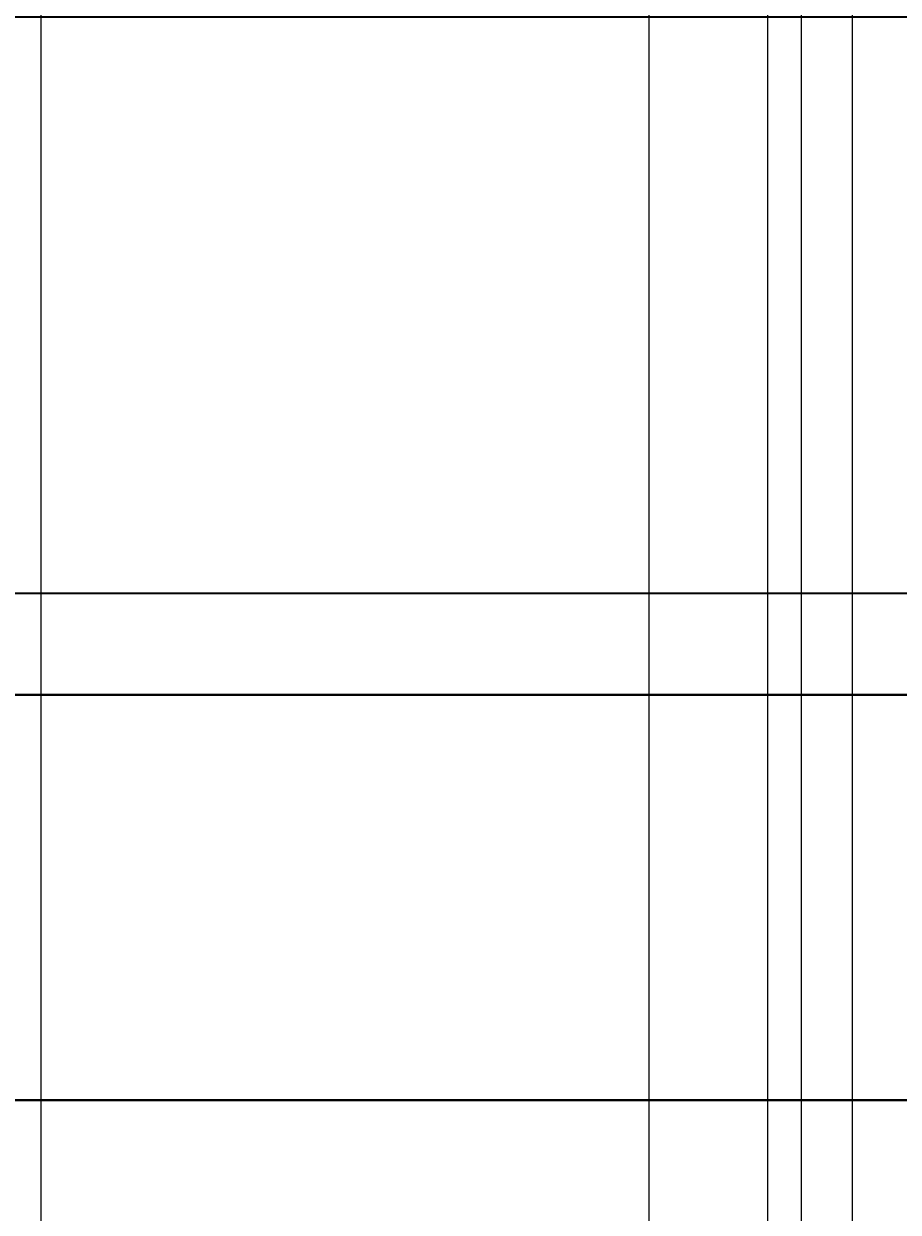
# Model space of a CAD drawing. Units: inches. Extents: x -6 to 289, y -8 to 323.
# Tile 63 of 107: x 212 to 238, y 124 to 159. Entities that reach past the tile are written whole.
import ezdxf

# ---------------------------------------------------------------- set-up
doc = ezdxf.new("R2010")
doc.units = ezdxf.units.IN
doc.header["$MEASUREMENT"] = 0
doc.layers.add('A-ANNO-DIMS', color=2, linetype='Continuous', lineweight=18)
doc.layers.add('A-ELEV', color=7, linetype='Continuous', lineweight=35)
doc.styles.get("Standard").update_dxf_attribs({"font": 'arial.ttf'})
doc.dimstyles.get("Standard").update_dxf_attribs({"dimtxt": 0.18, "dimasz": 0.18, "dimexe": 0.18, "dimexo": 0.0625, "dimgap": 0.09, "dimtad": 0, "dimtih": 1, "dimtoh": 1, "dimdec": 4, "dimzin": 0, "dimdsep": 46, "dimtxsty": 'Standard', "dimcen": 0.09, "dimadec": 0, "dimazin": 0, "dimtfac": 1, "dimtdec": 4, "dimtofl": 0, "dimtmove": 0, "dimatfit": 3, "dimfxl": 1, "dimtolj": 1, "dimtzin": 0, "dimarcsym": 0})

# ---------------------------------------------------------------- blocks, each defined once
blk = doc.blocks.new('*D24')
at = {"layer": 'A-ANNO-DIMS', "color": 0, "lineweight": -2, "transparency": 16777216}
for p, q in [((126.946, 178.654), (288.653, 178.654)), ((288.473, 178.474), (288.473, 159.153)), ((288.473, 139.469), (288.473, 158.789)), ((259.226, 139.289), (288.653, 139.289))]:
    blk.add_line(p, q, dxfattribs=at)
at = {"layer": 'A-ANNO-DIMS', "color": 0, "transparency": 16777216}
for points in [[(288.443, 178.474), (288.503, 178.474), (288.473, 178.654)], [(288.443, 139.469), (288.503, 139.469), (288.473, 139.289)]]:
    blk.add_solid(points, dxfattribs=at)
at = {"layer": 'Defpoints', "color": 0, "transparency": 16777216}
for p in [(126.883, 178.654), (288.473, 178.654), (259.164, 139.289)]:
    blk.add_point(p, dxfattribs=at)
at = {"layer": 'A-ANNO-DIMS', "color": 0, "transparency": 16777216, "insert": (288.473, 158.971), "char_height": 0.18, "attachment_point": 5}
blk.add_mtext('\\A1;39.365', dxfattribs=at)
blk = doc.blocks.new('*D43')
at = {"layer": 'A-ANNO-DIMS', "color": 0, "lineweight": -2, "transparency": 16777216}
for p, q in [((211.292, 224.326), (211.292, -8.391)), ((212.292, 224.326), (212.292, -8.391)), ((211.472, -8.211), (211.669, -8.211)), ((212.112, -8.211), (211.915, -8.211))]:
    blk.add_line(p, q, dxfattribs=at)
at = {"layer": 'A-ANNO-DIMS', "color": 0, "transparency": 16777216}
for points in [[(211.472, -8.181), (211.472, -8.241), (211.292, -8.211)], [(212.112, -8.181), (212.112, -8.241), (212.292, -8.211)]]:
    blk.add_solid(points, dxfattribs=at)
at = {"layer": 'Defpoints', "color": 0, "transparency": 16777216}
for p in [(211.292, 224.389), (212.292, 224.389), (212.292, -8.211)]:
    blk.add_point(p, dxfattribs=at)
at = {"layer": 'A-ANNO-DIMS', "color": 0, "transparency": 16777216, "insert": (211.792, -8.211), "char_height": 0.18, "attachment_point": 5}
blk.add_mtext('\\A1;1', dxfattribs=at)
blk = doc.blocks.new('*D44')
at = {"layer": 'A-ANNO-DIMS', "color": 0, "lineweight": -2, "transparency": 16777216}
for p, q in [((212.292, 224.326), (212.292, -8.391)), ((233.792, 224.326), (233.792, -8.391)), ((212.472, -8.211), (222.716, -8.211)), ((233.612, -8.211), (223.368, -8.211))]:
    blk.add_line(p, q, dxfattribs=at)
at = {"layer": 'A-ANNO-DIMS', "color": 0, "transparency": 16777216}
for points in [[(212.472, -8.181), (212.472, -8.241), (212.292, -8.211)], [(233.612, -8.181), (233.612, -8.241), (233.792, -8.211)]]:
    blk.add_solid(points, dxfattribs=at)
at = {"layer": 'Defpoints', "color": 0, "transparency": 16777216}
for p in [(212.292, 224.389), (233.792, 224.389), (233.792, -8.211)]:
    blk.add_point(p, dxfattribs=at)
at = {"layer": 'A-ANNO-DIMS', "color": 0, "transparency": 16777216, "insert": (223.042, -8.211), "char_height": 0.18, "attachment_point": 5}
blk.add_mtext('\\A1;21.5', dxfattribs=at)
blk = doc.blocks.new('*D45')
at = {"layer": 'A-ANNO-DIMS', "color": 0, "lineweight": -2, "transparency": 16777216}
for p, q in [((234.792, 225.326), (234.792, -8.391)), ((233.792, 224.326), (233.792, -8.391)), ((233.972, -8.211), (234.169, -8.211)), ((234.612, -8.211), (234.415, -8.211))]:
    blk.add_line(p, q, dxfattribs=at)
at = {"layer": 'A-ANNO-DIMS', "color": 0, "transparency": 16777216}
for points in [[(233.972, -8.181), (233.972, -8.241), (233.792, -8.211)], [(234.612, -8.181), (234.612, -8.241), (234.792, -8.211)]]:
    blk.add_solid(points, dxfattribs=at)
at = {"layer": 'Defpoints', "color": 0, "transparency": 16777216}
for p in [(234.792, 225.389), (233.792, 224.389), (234.792, -8.211)]:
    blk.add_point(p, dxfattribs=at)
at = {"layer": 'A-ANNO-DIMS', "color": 0, "transparency": 16777216, "insert": (234.292, -8.211), "char_height": 0.18, "attachment_point": 5}
blk.add_mtext('\\A1;1', dxfattribs=at)
blk = doc.blocks.new('*D46')
at = {"layer": 'A-ANNO-DIMS', "color": 0, "lineweight": -2, "transparency": 16777216}
for p, q in [((236.292, 226.826), (236.292, -8.391)), ((234.792, 225.326), (234.792, -8.391)), ((234.972, -8.211), (235.296, -8.211)), ((236.112, -8.211), (235.788, -8.211))]:
    blk.add_line(p, q, dxfattribs=at)
at = {"layer": 'A-ANNO-DIMS', "color": 0, "transparency": 16777216}
for points in [[(234.972, -8.181), (234.972, -8.241), (234.792, -8.211)], [(236.112, -8.181), (236.112, -8.241), (236.292, -8.211)]]:
    blk.add_solid(points, dxfattribs=at)
at = {"layer": 'Defpoints', "color": 0, "transparency": 16777216}
for p in [(236.292, 226.889), (234.792, 225.389), (236.292, -8.211)]:
    blk.add_point(p, dxfattribs=at)
at = {"layer": 'A-ANNO-DIMS', "color": 0, "transparency": 16777216, "insert": (235.542, -8.211), "char_height": 0.18, "attachment_point": 5}
blk.add_mtext('\\A1;1.5', dxfattribs=at)
blk = doc.blocks.new('*D80')
at = {"layer": 'A-ANNO-DIMS', "color": 0, "lineweight": -2, "transparency": 16777216}
for p, q in [((188.292, 116.842), (188.292, 322.969)), ((230.292, 116.842), (230.292, 322.969)), ((188.472, 322.789), (209.07, 322.789)), ((230.112, 322.789), (209.513, 322.789))]:
    blk.add_line(p, q, dxfattribs=at)
at = {"layer": 'A-ANNO-DIMS', "color": 0, "transparency": 16777216}
for points in [[(188.472, 322.819), (188.472, 322.759), (188.292, 322.789)], [(230.112, 322.819), (230.112, 322.759), (230.292, 322.789)]]:
    blk.add_solid(points, dxfattribs=at)
at = {"layer": 'Defpoints', "color": 0, "transparency": 16777216}
for p in [(230.292, 322.789), (188.292, 116.779), (230.292, 116.779)]:
    blk.add_point(p, dxfattribs=at)
at = {"layer": 'A-ANNO-DIMS', "color": 0, "transparency": 16777216, "insert": (209.292, 322.789), "char_height": 0.18, "attachment_point": 5}
blk.add_mtext('\\A1;42', dxfattribs=at)
blk = doc.blocks.new('*D81')
at = {"layer": 'A-ANNO-DIMS', "color": 0, "lineweight": -2, "transparency": 16777216}
for p, q in [((230.292, 68.842), (230.292, 322.969)), ((245.215, 66.286), (245.215, 322.969)), ((230.472, 322.789), (237.298, 322.789)), ((245.035, 322.789), (238.208, 322.789))]:
    blk.add_line(p, q, dxfattribs=at)
at = {"layer": 'A-ANNO-DIMS', "color": 0, "transparency": 16777216}
for points in [[(230.472, 322.819), (230.472, 322.759), (230.292, 322.789)], [(245.035, 322.819), (245.035, 322.759), (245.215, 322.789)]]:
    blk.add_solid(points, dxfattribs=at)
at = {"layer": 'Defpoints', "color": 0, "transparency": 16777216}
for p in [(245.215, 322.789), (230.292, 68.779), (245.215, 66.224)]:
    blk.add_point(p, dxfattribs=at)
at = {"layer": 'A-ANNO-DIMS', "color": 0, "transparency": 16777216, "insert": (237.753, 322.789), "char_height": 0.18, "attachment_point": 5}
blk.add_mtext('\\A1;14.923', dxfattribs=at)

msp = doc.modelspace()

# ---------------------------------------------------------------- linework, layer by layer
at = {"layer": 'A-ELEV'}
for p, q in [((115.1638, 139.2888), (259.1638, 139.2888)), ((259.1638, 127.2888), (115.1638, 127.2888)), ((115.1638, 127.2888), (259.1638, 127.2888))]:
    msp.add_line(p, q, dxfattribs=at)
for points in [[(247.1638, 139.2888), (115.1638, 139.2888), (115.1638, 162.3484), (247.1638, 162.3484)], [(244.1638, 142.2888), (118.1638, 142.2888), (118.1638, 159.3484), (244.1638, 159.3484)]]:
    msp.add_lwpolyline(points, close=True, dxfattribs=at)

# ---------------------------------------------------------------- dimensions: what is measured, and where the dimension line sits
at = {"layer": 'A-ANNO-DIMS'}
for base, p1, p2, override, picture, middle in [((230.2918, 322.7888), (188.2918, 116.7795), (230.2918, 116.7795), {"dimdec": 0, "dimlfac": 1, "dimrnd": 0, "dimzin": 0, "dimdsep": 46, "dimlunit": 2}, '*D80', (209.2918, 322.7888)), ((245.2146, 322.7888), (230.2918, 68.7795), (245.2146, 66.2238), {"dimdec": 3, "dimlfac": 1, "dimrnd": 0, "dimzin": 0, "dimdsep": 46, "dimlunit": 2}, '*D81', (237.7532, 322.7888)), ((236.2918, -8.2112), (234.7918, 225.3887), (236.2918, 226.8887), {"dimdec": 1, "dimlfac": 1, "dimrnd": 0, "dimzin": 0, "dimdsep": 46, "dimlunit": 2}, '*D46', (235.5418, -8.2112)), ((234.7918, -8.2112), (233.7918, 224.3887), (234.7918, 225.3887), {"dimdec": 0, "dimlfac": 1, "dimrnd": 0, "dimzin": 0, "dimdsep": 46, "dimlunit": 2}, '*D45', (234.2918, -8.2112)), ((212.2918, -8.2112), (211.2918, 224.3887), (212.2918, 224.3887), {"dimdec": 0, "dimlfac": 1, "dimrnd": 0, "dimzin": 0, "dimdsep": 46, "dimlunit": 2}, '*D43', (211.7918, -8.2112)), ((233.7918, -8.2112), (212.2918, 224.3887), (233.7918, 224.3887), {"dimdec": 1, "dimlfac": 1, "dimrnd": 0, "dimzin": 0, "dimdsep": 46, "dimlunit": 2}, '*D44', (223.0418, -8.2112))]:
    dim = msp.add_linear_dim(base=base, p1=p1, p2=p2, dimstyle='Standard', override=override, dxfattribs=at)
    dim.commit()
    dim.dimension.update_dxf_attribs({"geometry": picture, "text_midpoint": middle})
dim = msp.add_linear_dim(base=(288.4733, 178.654), p1=(259.1638, 139.2888), p2=(126.8835, 178.654), angle=90, dimstyle='Standard', override={"dimdec": 3, "dimlfac": 1, "dimrnd": 0, "dimzin": 0, "dimdsep": 46, "dimlunit": 2}, dxfattribs=at)
dim.commit()
dim.dimension.update_dxf_attribs({"geometry": '*D24', "text_midpoint": (288.4733, 158.9714)})

doc.saveas('drawing.dxf')
